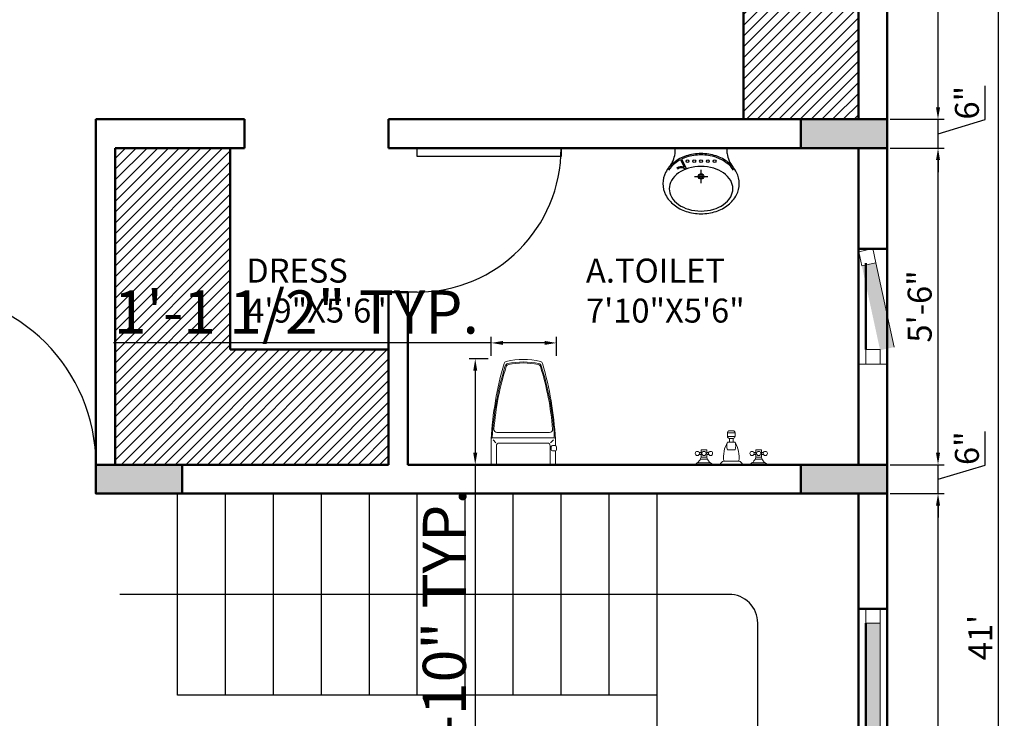
# Model space of a CAD drawing. Units: inches. Extents: x 3064 to 19385, y 846 to 15425.
# Tile 44 of 108: x 5352 to 5557, y 1129 to 1275. Entities that reach past the tile are written whole.
import ezdxf

# ---------------------------------------------------------------- set-up
doc = ezdxf.new("R2010")
doc.units = ezdxf.units.IN
for name, color, linetype, lineweight in [('A-ANNO-DIMS', 2, 'Continuous', 18), ('A-AREA-IDEN', 3, 'Continuous', 18), ('A-COLS', 1, 'Continuous', 35), ('A-DOOR', 3, 'Continuous', 25), ('A-FLOR-FIXT', 9, 'Continuous', 18), ('A-FLOR-STRS', 2, 'Continuous', 25), ('A-FURN-PATT', 252, 'Continuous', 13), ('A-GLAZ', 4, 'Continuous', 18), ('A-WALL', 7, 'Continuous', 50)]:
    doc.layers.add(name, color=color, linetype=linetype, lineweight=lineweight)
doc.layers.add('THIET-BI', color=21, linetype='Continuous')
doc.styles.get("Standard").update_dxf_attribs({"font": 'arial.ttf'})
doc.dimstyles.new('ISO-25', dxfattribs={"dimtxt": 9, "dimasz": 2.5, "dimexe": 1.25, "dimexo": 0.625, "dimtad": 1, "dimdec": 1, "dimlunit": 3, "dimtxsty": 'Standard', "dimcen": 2.5, "dimadec": 0, "dimazin": 0, "dimtfac": 1, "dimtdec": 1, "dimtmove": 0, "dimatfit": 3, "dimfxl": 1, "dimarcsym": 0})
pattern_1 = [(45, (848.524, -4.2436), (-1.122532, 1.122532), [])]

# ---------------------------------------------------------------- blocks, each defined once
blk = doc.blocks.new('*U3')
for p, q in [((0, 0), (0, -6)), ((36, 0), (36, -6))]:
    blk.add_line(p, q)
blk.add_lwpolyline([(0, 0), (0, 36), (1.75, 36), (1.75, 0)], close=True)
blk.add_arc((0, 0), 36, 0, 90)
blk = doc.blocks.new('*U4')
for p, q in [((0, 0), (0, -6)), ((30, 0), (30, -6))]:
    blk.add_line(p, q)
blk.add_lwpolyline([(0, 0), (0, 30), (1.75, 30), (1.75, 0)], close=True)
blk.add_arc((0, 0), 30, 0, 90)
blk = doc.blocks.new('A$C430D11A0')
at = {"layer": 'THIET-BI'}
for p, q in [((90, 445), (90, 485)), ((475, 485), (90, 485)), ((475, 483), (90, 483)), ((475, 445), (475, 485)), ((129.4, 398.5), (158.2, 344.4)), ((138.3, 403), (176, 332.4)), ((282.5, 226.2), (282.5, 324.8)), ((233.4, 275.5), (331.9, 275.5))]:
    blk.add_line(p, q, dxfattribs=at)
for points in [[(565, 222.5, 0.121635), (544.7, 304.8, 0.10526), (482.3, 379.8, 0.088175), (393.4, 427.4, 0.079002), (282.5, 445, 0.079002), (171.6, 427.4, 0.088175), (82.7, 379.8, 0.10526), (20.3, 304.8, 0.121635), (0, 222.5, 0.121635), (20.3, 140.2, 0.10526), (82.7, 65.2, 0.088175), (171.6, 17.6, 0.079002), (282.5, 0, 0.079002), (393.4, 17.6, 0.088175), (482.3, 65.2, 0.10526), (544.7, 140.2, 0.121635)], [(517.5, 185, 0.134042), (501.2, 244.9, 0.106817), (448.7, 301.7, 0.082468), (375.6, 336.7, 0.070874), (282.5, 350, 0.070874), (189.4, 336.7, 0.082468), (116.3, 301.7, 0.106817), (63.8, 244.9, 0.134042), (47.5, 185, 0.134042), (63.8, 125.1, 0.106817), (116.3, 68.3, 0.082468), (189.4, 33.3, 0.070874), (282.5, 20, 0.070874), (375.6, 33.3, 0.082468), (448.7, 68.3, 0.106817), (501.2, 125.1, 0.134042)]]:
    blk.add_lwpolyline(points, format="xyb", close=True, dxfattribs=at)
for points in [[(129.4, 398.5, 0.043566), (88.9, 372, 0.07708), (42.1, 321.6, 0.041486)], [(522.9, 321.6, 0.07708), (476.1, 372, 0.088175), (390.3, 417.9, 0.079002), (282.5, 435, 0.079002), (174.7, 417.9, 0.035427), (138.3, 403, 0.07708)]]:
    blk.add_lwpolyline(points, format="xyb", dxfattribs=at)
for centre, radius in [((182.5, 388.2), 10.5), ((232.5, 388.2), 10.5), ((282.5, 388.2), 10.5), ((332.5, 388.2), 10.5), ((382.5, 388.2), 10.5), ((282.5, 275.5), 20), ((282.5, 275.5), 15)]:
    blk.add_circle(centre, radius, dxfattribs=at)
for centre, radius, start, end in [((-103.8, 468.9), 195.3, 320.8253, 352.95569), ((668.8, 468.9), 195.3, 187.04431, 219.1747), ((136.4, 285.4), 62.9, 69.64296, 123.47738), ((136.4, 285.4), 52.9, 55.24551, 123.47738)]:
    blk.add_arc(centre, radius, start, end, dxfattribs=at)
blk = doc.blocks.new('WC-P05')
for p, q in [((-202.4, 531.6), (-202.4, 439.1)), ((-192.4, 541.6), (262.6, 541.6)), ((-163.4, 541.6), (-163.4, 400.6)), ((233.6, 541.6), (233.6, 400.6)), ((272.6, 531.6), (272.6, 351.6)), ((-201.4, 439.1), (-180.4, 439.1)), ((-210.4, 430.1), (-210.4, 409.1)), ((-202.4, 400.1), (-202.4, 351.6)), ((-201.4, 400.1), (-180.4, 400.1)), ((-166.9, 378.6), (-188.2, 357.3)), ((-171.4, 430.1), (-171.4, 409.1)), ((-143.4, 380.6), (213.6, 380.6)), ((237.1, 378.6), (258.4, 357.3)), ((-192.4, 341.6), (262.6, 341.6)), ((-159.3, 302.6), (229.5, 302.6))]:
    blk.add_line(p, q)
blk.add_lwpolyline([(-90.9, -221.9, 0.114547), (161, -222, 0.114547)], format="xyb")
for centre, radius, start, end in [((-192.4, 531.6), 10, 90, 180), ((262.6, 531.6), 10, 0, 90), ((-201.4, 430.1), 9, 90, 180), ((-180.4, 430.1), 9, 0, 90), ((-201.4, 409.1), 9, 180, 270), ((-180.4, 409.1), 9, 270, 0), ((-143.4, 400.6), 20, 180, 270), ((213.6, 400.6), 20, 270, 0), ((2308.9, 492.3), 2515.2, 183.20675, 196.12415), ((-192.4, 351.6), 10, 180, 270), ((1906, 447.2), 2102.6, 182.87428, 197.65536), ((-159.3, 280.1), 22.5, 90, 184.62462), ((-1835.8, 447.2), 2102.6, 342.34464, 357.12572), ((-2238.7, 492.3), 2515.2, 343.87268, 356.79325), ((229.5, 280.1), 22.5, 355.37538, 90), ((262.6, 351.6), 10, 270, 0), ((1905.9, 447.2), 2094.5, 184.62454, 197.52765), ((-1835.8, 447.2), 2094.6, 342.46396, 355.37538), ((-85.8, -199.9), 22.5, 196.12415, 256.89941), ((-76.1, -183.7), 22.5, 197.65536, 257.50587), ((-69.9, -176.8), 22.5, 197.52765, 258.10049), ((35.1, 318), 536.4, 257.50587, 282.49413), ((35.7, 324.3), 534.7, 258.10049, 281.73735), ((139.9, -177.1), 22.5, 281.73735, 342.46396), ((146.2, -183.7), 22.5, 282.49413, 342.34464), ((155.9, -200.1), 22.5, 283.03778, 343.87268)]:
    blk.add_arc(centre, radius, start, end)
blk = doc.blocks.new('Faucet - Bathroom front')
for p, q in [((-0.5, 4.25), (0.5, 4.25)), ((0.5, 3.75), (-0.5, 3.75)), ((-0.5, 3), (0.5, 3)), ((-0.25, 3), (-0.25, 3.5)), ((0.25, 3.5), (0.25, 3)), ((-4, 1.625), (-4.25, 1.625)), ((-4, 1.375), (-4.25, 1.375)), ((-3.25, 1.625), (-3, 1.625)), ((-3.25, 1.375), (-3, 1.375)), ((0.5, 2), (-0.5, 2)), ((3.25, 1.625), (3, 1.625)), ((3.25, 1.375), (3, 1.375)), ((4, 1.625), (4.25, 1.625)), ((4, 1.375), (4.25, 1.375)), ((-5, 0), (-2.25, 0)), ((-4.5087, 0.25), (-2.7408, 0.25)), ((-3.1442, 0.75), (-4.0979, 0.75)), ((-1.5, 0), (1.5, 0)), ((-1, 0.5), (1, 0.5)), ((2.25, 0), (5, 0)), ((2.7413, 0.25), (4.5092, 0.25)), ((4.1058, 0.75), (3.1521, 0.75))]:
    blk.add_line(p, q)
for points in [[(-0.5, 3.75), (-0.5, 4.25)], [(-0.25, 4.5), (0.25, 4.5)], [(0.5, 4.25), (0.5, 3.75)], [(0.25, 3.5), (-0.25, 3.5)]]:
    blk.add_lwpolyline(points)
for points in [[(-4, 1), (-4, 2), (-3.25, 2), (-3.25, 1)], [(3.25, 1), (3.25, 2), (4, 2), (4, 1)]]:
    blk.add_lwpolyline(points, close=True)
for centre in [(-4.5, 1.5), (-3.625, 1.5), (-2.75, 1.5), (2.75, 1.5), (3.625, 1.5), (4.5, 1.5)]:
    blk.add_circle(centre, 0.2795)
for centre, radius, start, end in [((-0.2575, 4.2575), 0.2426, 88.22243, 181.7776), ((0.2575, 4.2575), 0.2426, 358.2224, 91.77757), ((3, 1), 4.0311, 150.2551, 187.125), ((0.6413, 2.5), 1.246, 156.3417, 203.6583), ((-0.2575, 3.7425), 0.2426, 178.2224, 271.7776), ((0.2575, 3.7425), 0.2426, 268.2224, 1.777565), ((-3, 1), 4.0311, 352.875, 29.74488), ((-0.6413, 2.5), 1.246, 336.3417, 23.65835), ((-5.375, 1.375), 1.4252, 285.2551, 344.7449), ((-1.875, 1.375), 1.4252, 195.2551, 254.7449), ((-0.7962, -0.2038), 0.7327, 106.1502, 163.8498), ((0.7962, -0.2038), 0.7327, 16.1502, 73.84979), ((1.875, 1.375), 1.4252, 285.2551, 344.7449), ((5.375, 1.375), 1.4252, 195.2551, 254.7449)]:
    blk.add_arc(centre, radius, start, end)
blk = doc.blocks.new('*D82')
at = {"layer": 'A-ANNO-DIMS', "color": 0, "lineweight": -2, "transparency": 16777216}
for p, q in [((5533.64, 1176.1), (5544.85, 1176.1)), ((5543.6, 980.6), (5543.6, 1173.6)), ((5527.64, 978.1), (5544.85, 978.1))]:
    blk.add_line(p, q, dxfattribs=at)
at = {"layer": 'A-ANNO-DIMS', "color": 0, "transparency": 16777216}
for points in [[(5543.18, 1173.6), (5544.02, 1173.6), (5543.6, 1176.1)], [(5543.18, 980.6), (5544.02, 980.6), (5543.6, 978.1)]]:
    blk.add_solid(points, dxfattribs=at)
at = {"layer": 'Defpoints', "color": 0, "transparency": 16777216}
for p in [(5533.02, 1176.1), (5543.6, 1176.1), (5527.02, 978.1)]:
    blk.add_point(p, dxfattribs=at)
at = {"layer": 'A-ANNO-DIMS', "color": 0, "transparency": 16777216, "insert": (5540.42, 1077.1), "char_height": 5, "attachment_point": 5, "rotation": 90}
blk.add_mtext('16\'-6"', dxfattribs=at)
blk = doc.blocks.new('*D83')
at = {"layer": 'A-ANNO-DIMS', "color": 0, "lineweight": -2, "transparency": 16777216}
for p, q in [((5553.45, 1182.05), (5553.45, 1189.07)), ((5543.6, 1184.6), (5543.6, 1187.1)), ((5533.64, 1182.1), (5544.85, 1182.1)), ((5543.6, 1176.1), (5543.6, 1182.1)), ((5543.6, 1176.1), (5543.6, 1182.1)), ((5543.6, 1179.1), (5553.45, 1182.05)), ((5533.64, 1176.1), (5544.85, 1176.1)), ((5543.6, 1173.6), (5543.6, 1171.1))]:
    blk.add_line(p, q, dxfattribs=at)
at = {"layer": 'A-ANNO-DIMS', "color": 0, "transparency": 16777216}
for points in [[(5543.18, 1184.6), (5544.02, 1184.6), (5543.6, 1182.1)], [(5543.18, 1173.6), (5544.02, 1173.6), (5543.6, 1176.1)]]:
    blk.add_solid(points, dxfattribs=at)
at = {"layer": 'Defpoints', "color": 0, "transparency": 16777216}
for p in [(5533.02, 1182.1), (5543.6, 1182.1), (5533.02, 1176.1)]:
    blk.add_point(p, dxfattribs=at)
at = {"layer": 'A-ANNO-DIMS', "color": 0, "transparency": 16777216, "insert": (5550.27, 1185.56), "char_height": 5, "attachment_point": 5, "rotation": 90}
blk.add_mtext('6"', dxfattribs=at)
blk = doc.blocks.new('*D84')
at = {"layer": 'A-ANNO-DIMS', "color": 0, "lineweight": -2, "transparency": 16777216}
for p, q in [((5533.64, 1248.1), (5544.85, 1248.1)), ((5543.6, 1184.6), (5543.6, 1245.6)), ((5533.64, 1182.1), (5544.85, 1182.1))]:
    blk.add_line(p, q, dxfattribs=at)
at = {"layer": 'A-ANNO-DIMS', "color": 0, "transparency": 16777216}
for points in [[(5543.18, 1245.6), (5544.02, 1245.6), (5543.6, 1248.1)], [(5543.18, 1184.6), (5544.02, 1184.6), (5543.6, 1182.1)]]:
    blk.add_solid(points, dxfattribs=at)
at = {"layer": 'Defpoints', "color": 0, "transparency": 16777216}
for p in [(5533.02, 1248.1), (5543.6, 1248.1), (5533.02, 1182.1)]:
    blk.add_point(p, dxfattribs=at)
at = {"layer": 'A-ANNO-DIMS', "color": 0, "transparency": 16777216, "insert": (5540.42, 1215.1), "char_height": 5, "attachment_point": 5, "rotation": 90}
blk.add_mtext('5\'-6"', dxfattribs=at)
blk = doc.blocks.new('*D85')
at = {"layer": 'A-ANNO-DIMS', "color": 0, "lineweight": -2, "transparency": 16777216}
for p, q in [((5553.45, 1254.05), (5553.45, 1261.07)), ((5543.6, 1256.6), (5543.6, 1259.1)), ((5533.64, 1254.1), (5544.85, 1254.1)), ((5543.6, 1248.1), (5543.6, 1254.1)), ((5543.6, 1248.1), (5543.6, 1254.1)), ((5543.6, 1251.1), (5553.45, 1254.05)), ((5533.64, 1248.1), (5544.85, 1248.1)), ((5543.6, 1245.6), (5543.6, 1243.1))]:
    blk.add_line(p, q, dxfattribs=at)
at = {"layer": 'A-ANNO-DIMS', "color": 0, "transparency": 16777216}
for points in [[(5543.18, 1256.6), (5544.02, 1256.6), (5543.6, 1254.1)], [(5543.18, 1245.6), (5544.02, 1245.6), (5543.6, 1248.1)]]:
    blk.add_solid(points, dxfattribs=at)
at = {"layer": 'Defpoints', "color": 0, "transparency": 16777216}
for p in [(5533.02, 1254.1), (5543.6, 1254.1), (5533.02, 1248.1)]:
    blk.add_point(p, dxfattribs=at)
at = {"layer": 'A-ANNO-DIMS', "color": 0, "transparency": 16777216, "insert": (5550.27, 1257.56), "char_height": 5, "attachment_point": 5, "rotation": 90}
blk.add_mtext('6"', dxfattribs=at)
blk = doc.blocks.new('*D86')
at = {"layer": 'A-ANNO-DIMS', "color": 0, "lineweight": -2, "transparency": 16777216}
for p, q in [((5527.64, 1386.1), (5544.85, 1386.1)), ((5543.6, 1256.6), (5543.6, 1383.6)), ((5533.64, 1254.1), (5544.85, 1254.1))]:
    blk.add_line(p, q, dxfattribs=at)
at = {"layer": 'A-ANNO-DIMS', "color": 0, "transparency": 16777216}
for points in [[(5543.18, 1383.6), (5544.02, 1383.6), (5543.6, 1386.1)], [(5543.18, 1256.6), (5544.02, 1256.6), (5543.6, 1254.1)]]:
    blk.add_solid(points, dxfattribs=at)
at = {"layer": 'Defpoints', "color": 0, "transparency": 16777216}
for p in [(5527.02, 1386.1), (5543.6, 1386.1), (5533.02, 1254.1)]:
    blk.add_point(p, dxfattribs=at)
at = {"layer": 'A-ANNO-DIMS', "color": 0, "transparency": 16777216, "insert": (5540.46, 1320.1), "char_height": 5, "attachment_point": 5, "rotation": 90}
blk.add_mtext("11'", dxfattribs=at)
blk = doc.blocks.new('*D88')
at = {"layer": 'A-ANNO-DIMS', "color": 0, "lineweight": -2, "transparency": 16777216}
for p, q in [((5533.64, 1392.1), (5557.42, 1392.1)), ((5556.17, 1389.6), (5556.17, 902.6)), ((5533.64, 900.1), (5557.42, 900.1))]:
    blk.add_line(p, q, dxfattribs=at)
at = {"layer": 'A-ANNO-DIMS', "color": 0, "transparency": 16777216}
for points in [[(5555.75, 1389.6), (5556.59, 1389.6), (5556.17, 1392.1)], [(5555.75, 902.6), (5556.59, 902.6), (5556.17, 900.1)]]:
    blk.add_solid(points, dxfattribs=at)
at = {"layer": 'Defpoints', "color": 0, "transparency": 16777216}
for p in [(5533.02, 1392.1), (5533.02, 900.1), (5556.17, 900.1)]:
    blk.add_point(p, dxfattribs=at)
at = {"layer": 'A-ANNO-DIMS', "color": 0, "transparency": 16777216, "insert": (5553.04, 1146.1), "char_height": 5, "attachment_point": 5, "rotation": 90}
blk.add_mtext("41'", dxfattribs=at)
blk = doc.blocks.new('WIN-600')
h = blk.add_hatch(color=256)
h.dxf.hatch_style = 1
h.paths.add_polyline_path([(3, 18), (0, 18), (0, 0), (3, 0)])
blk.add_line((3, 18), (3, 0))
blk.add_lwpolyline([(3, 18), (0, 18), (0, 21), (3, 21)], close=True)
blk = doc.blocks.new('WIN-1800-PAIR')
h = blk.add_hatch(color=256)
h.dxf.hatch_style = 1
h.paths.add_polyline_path([(0, 0), (3, 0), (3, 70.5), (0, 70.5)])
h.paths.add_polyline_path([(3, 144), (0, 144), (0, 73.5), (3, 73.5)])
blk.add_line((3, 144), (3, 73.5))
blk.add_lwpolyline([(3, 144), (0, 144), (0, 147), (3, 147)], close=True)
blk = doc.blocks.new('*D405')
at = {"layer": 'A-ANNO-DIMS', "color": 0, "lineweight": -2, "transparency": 16777216}
for p, q in [((5449.79, 1204.19), (5445.85, 1204.19)), ((5447.1, 1201.69), (5447.1, 1184.6)), ((5449.79, 1182.1), (5445.85, 1182.1)), ((5447.1, 1182.1), (5447.1, 1091.69))]:
    blk.add_line(p, q, dxfattribs=at)
at = {"layer": 'A-ANNO-DIMS', "color": 0, "transparency": 16777216}
for points in [[(5446.69, 1201.69), (5447.52, 1201.69), (5447.1, 1204.19)], [(5446.69, 1184.6), (5447.52, 1184.6), (5447.1, 1182.1)]]:
    blk.add_solid(points, dxfattribs=at)
at = {"layer": 'Defpoints', "color": 0, "transparency": 16777216}
for p in [(5450.42, 1204.19), (5447.1, 1182.1), (5450.42, 1182.1)]:
    blk.add_point(p, dxfattribs=at)
at = {"layer": 'A-ANNO-DIMS', "color": 0, "transparency": 16777216, "insert": (5441.83, 1135.64), "char_height": 9, "attachment_point": 5, "rotation": 90}
blk.add_mtext('WC 1\'-10" TYP.', dxfattribs=at)
blk = doc.blocks.new('*D406')
at = {"layer": 'A-ANNO-DIMS', "color": 0, "lineweight": -2, "transparency": 16777216}
for p, q in [((5450.42, 1207.5), (5371.68, 1207.5)), ((5450.42, 1204.81), (5450.42, 1208.75)), ((5461.55, 1207.5), (5452.92, 1207.5)), ((5464.05, 1204.81), (5464.05, 1208.75))]:
    blk.add_line(p, q, dxfattribs=at)
at = {"layer": 'A-ANNO-DIMS', "color": 0, "transparency": 16777216}
for points in [[(5452.92, 1207.92), (5452.92, 1207.09), (5450.42, 1207.5)], [(5461.55, 1207.92), (5461.55, 1207.09), (5464.05, 1207.5)]]:
    blk.add_solid(points, dxfattribs=at)
at = {"layer": 'Defpoints', "color": 0, "transparency": 16777216}
for p in [(5450.42, 1207.5), (5450.42, 1204.19), (5464.05, 1204.19)]:
    blk.add_point(p, dxfattribs=at)
at = {"layer": 'A-ANNO-DIMS', "color": 0, "transparency": 16777216, "insert": (5409.8, 1212.78), "char_height": 9, "attachment_point": 5}
blk.add_mtext('1\'-1 1/2" TYP.', dxfattribs=at)

msp = doc.modelspace()

# ---------------------------------------------------------------- hatches: boundary and pattern name
at = {"layer": 'A-COLS'}
h = msp.add_hatch(color=256, dxfattribs=at)
h.dxf.hatch_style = 1
h.paths.add_polyline_path([(5533.02, 1254.1), (5515.02, 1254.1), (5515.02, 1248.1), (5533.02, 1248.1)])
h = msp.add_hatch(color=256, dxfattribs=at)
h.dxf.hatch_style = 1
h.paths.add_polyline_path([(5386.02, 1182.1), (5368.02, 1182.1), (5368.02, 1176.1), (5386.02, 1176.1)])
h = msp.add_hatch(color=256, dxfattribs=at)
h.dxf.hatch_style = 1
h.paths.add_polyline_path([(5533.02, 1182.1), (5515.02, 1182.1), (5515.02, 1176.1), (5533.02, 1176.1)])
at = {"layer": 'A-FURN-PATT'}
h = msp.add_hatch(dxfattribs=at)
h.set_pattern_fill('ANSI31', color=256, scale=0.5)
h.set_pattern_definition(pattern_1)
h.paths.add_polyline_path([(5503.02, 1254.1), (5527.02, 1254.1), (5527.02, 1386.1), (5503.02, 1386.1)])
h = msp.add_hatch(dxfattribs=at)
h.set_pattern_fill('ANSI31', color=256, scale=0.5)
h.set_pattern_definition(pattern_1)
h.paths.add_polyline_path([(5396.02, 1206.1), (5396.02, 1248.1), (5372.02, 1248.1), (5372.02, 1182.1), (5386.02, 1182.1), (5429.02, 1182.1), (5429.02, 1206.1)])

# ---------------------------------------------------------------- linework, layer by layer
at = {"layer": 'A-FLOR-STRS'}
for p, q in [((5385.02, 1134.1), (5385.02, 1176.1)), ((5395.02, 1134.1), (5395.02, 1176.1)), ((5405.02, 1134.1), (5405.02, 1176.1)), ((5415.02, 1134.1), (5415.02, 1176.1)), ((5425.02, 1134.1), (5425.02, 1176.1)), ((5435.02, 1134.1), (5435.02, 1176.1)), ((5445.02, 1134.1), (5445.02, 1176.1)), ((5455.02, 1134.1), (5455.02, 1176.1)), ((5465.02, 1134.1), (5465.02, 1176.1)), ((5475.02, 1134.1), (5475.02, 1176.1)), ((5485.02, 1020.1), (5485.02, 1176.1)), ((5485.02, 1134.1), (5385.02, 1134.1))]:
    msp.add_line(p, q, dxfattribs=at)
msp.add_lwpolyline([(5392.51, 999.1), (5500.02, 999.1, 0.414214), (5506.02, 1005.1), (5506.02, 1149.1, 0.414214), (5500.02, 1155.1), (5373.02, 1155.1)], format="xyb", dxfattribs=at)
at = {"layer": 'A-GLAZ'}
msp.add_line((5527.02, 1203.1), (5533.02, 1203.1), dxfattribs=at)
msp.add_lwpolyline([(5531.52, 1203.1), (5528.52, 1203.1), (5528.52, 1206.1), (5531.52, 1206.1)], close=True, dxfattribs=at)
at = {"layer": 'A-WALL'}
for p, q in [((5533.02, 900.1), (5533.02, 1392.1)), ((5503.02, 1254.1), (5503.02, 1386.1)), ((5527.02, 1254.1), (5527.02, 1386.1)), ((5399.02, 1254.1), (5368.02, 1254.1)), ((5368.02, 1254.1), (5368.02, 1176.1)), ((5399.02, 1254.1), (5399.02, 1248.1)), ((5527.02, 1254.1), (5429.02, 1254.1)), ((5429.02, 1254.1), (5429.02, 1248.1)), ((5399.02, 1248.1), (5372.02, 1248.1)), ((5372.02, 1248.1), (5372.02, 1182.1)), ((5396.02, 1248.1), (5396.02, 1206.1)), ((5527.02, 1248.1), (5429.02, 1248.1)), ((5527.02, 1182.1), (5527.02, 1248.1)), ((5527.02, 1227.1), (5533.02, 1227.1)), ((5528.52, 1224.1), (5528.52, 1206.1)), ((5433.02, 1218.1), (5429.02, 1218.1)), ((5429.02, 1218.1), (5429.02, 1182.1)), ((5433.02, 1182.1), (5433.02, 1218.1)), ((5429.02, 1206.1), (5396.02, 1206.1)), ((5429.02, 1182.1), (5372.02, 1182.1)), ((5527.02, 1182.1), (5433.02, 1182.1)), ((5527.02, 1176.1), (5368.02, 1176.1)), ((5527.02, 978.1), (5527.02, 1176.1)), ((5533.02, 1152.1), (5527.02, 1152.1)), ((5528.52, 1149.1), (5528.52, 1078.6))]:
    msp.add_line(p, q, dxfattribs=at)
for points in [[(5533.02, 1254.1), (5515.02, 1254.1), (5515.02, 1248.1), (5533.02, 1248.1)], [(5386.02, 1182.1), (5368.02, 1182.1), (5368.02, 1176.1), (5386.02, 1176.1)], [(5533.02, 1182.1), (5515.02, 1182.1), (5515.02, 1176.1), (5533.02, 1176.1)]]:
    msp.add_lwpolyline(points, close=True, dxfattribs=at)

# ---------------------------------------------------------------- block references
at = {"layer": 'A-DOOR', "rotation": 270}
msp.add_blockref('*U4', (5435.02, 1248.1), dxfattribs=at)
at = {"layer": 'A-DOOR'}
msp.add_blockref('*U3', (5332.02, 1182.1), dxfattribs=at)
at = {"layer": 'A-FLOR-FIXT'}
for name, p, xscale, yscale, zscale in [('A$C430D11A0', (5486.22, 1234.41), 0.0282220760332506, 0.0282220760332506, 0.0282220760332506), ('Faucet - Bathroom front', (5500.49, 1182.1), 1.573166238287219, 1.573166238287219, 1.573166238287219)]:
    msp.add_blockref(name, p, dxfattribs=dict(at, xscale=xscale, yscale=yscale, zscale=zscale))
at = {"layer": 'A-FLOR-FIXT', "xscale": 0.0282220760332506, "yscale": 0.0282220760332506, "zscale": 0.0282220760332506, "rotation": 180}
msp.add_blockref('WC-P05', (5458.11, 1197.38), dxfattribs=at)
at = {"layer": 'A-GLAZ', "rotation": 12.21571913413076}
msp.add_blockref('WIN-600', (5531.52, 1205.99), dxfattribs=at)
at = {"layer": 'A-GLAZ'}
msp.add_blockref('WIN-1800-PAIR', (5528.52, 1005.1), dxfattribs=at)

# ---------------------------------------------------------------- texts
at = {"layer": 'A-AREA-IDEN', "char_height": 5, "attachment_point": 1}
for s, insert in [('DRESS\\P4\'9"X5\'6"', (5399.35, 1225.07)), ('A.TOILET\\P7\'10"X5\'6"', (5470.19, 1225.07))]:
    msp.add_mtext_dynamic_manual_height_columns(s, width=67.5924, gutter_width=12.5, heights=[0], dxfattribs=dict(at, insert=insert))

# ---------------------------------------------------------------- dimensions: what is measured, and where the dimension line sits
at = {"layer": 'A-ANNO-DIMS'}
for base, p1, p2, override, picture, middle in [((5556.17, 900.1), (5533.02, 1392.1), (5533.02, 900.1), {"dimtxt": 5, "dimclrd": 0, "dimclre": 0, "dimclrt": 0}, '*D88', (5553.04, 1146.1)), ((5543.6, 1386.1), (5533.02, 1254.1), (5527.02, 1386.1), {"dimtxt": 5, "dimclrd": 0, "dimclre": 0, "dimclrt": 0, "dimtmove": 1}, '*D86', (5540.46, 1320.1)), ((5543.6, 1254.1), (5533.02, 1248.1), (5533.02, 1254.1), {"dimtxt": 5, "dimclrd": 0, "dimclre": 0, "dimclrt": 0, "dimtmove": 1}, '*D85', (5550.27, 1254.68)), ((5543.6, 1248.1), (5533.02, 1182.1), (5533.02, 1248.1), {"dimtxt": 5, "dimclrd": 0, "dimclre": 0, "dimclrt": 0, "dimtmove": 1}, '*D84', (5540.42, 1215.1)), ((5543.6, 1182.1), (5533.02, 1176.1), (5533.02, 1182.1), {"dimtxt": 5, "dimclrd": 0, "dimclre": 0, "dimclrt": 0, "dimtmove": 1}, '*D83', (5550.27, 1182.68)), ((5543.6, 1176.1), (5527.02, 978.1), (5533.02, 1176.1), {"dimtxt": 5, "dimclrd": 0, "dimclre": 0, "dimclrt": 0, "dimtmove": 1}, '*D82', (5540.42, 1077.1))]:
    dim = msp.add_linear_dim(base=base, p1=p1, p2=p2, angle=90, dimstyle='ISO-25', override=override, dxfattribs=at)
    dim.commit()
    dim.dimension.update_dxf_attribs({"geometry": picture, "text_midpoint": middle})
for base, p1, p2, angle, text, picture, middle in [((5450.42, 1207.5), (5464.05, 1204.19), (5450.42, 1204.19), 180, '<> TYP.', '*D406', (5409.8, 1212.78)), ((5447.1, 1182.1), (5450.42, 1204.19), (5450.42, 1182.1), 270, 'WC <> TYP.', '*D405', (5441.83, 1135.64))]:
    dim = msp.add_linear_dim(base=base, p1=p1, p2=p2, angle=angle, text=text, dimstyle='ISO-25', override={"dimdec": 1, "dimrnd": 0, "dimzin": 1, "dimlunit": 4, "dimfrac": 2}, dxfattribs=at)
    dim.commit()
    dim.dimension.update_dxf_attribs({"geometry": picture, "text_midpoint": middle})

doc.saveas('drawing.dxf')
